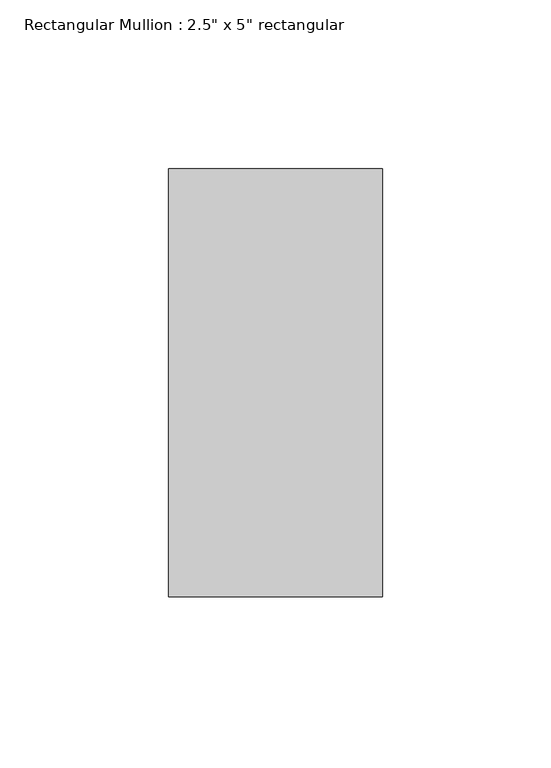
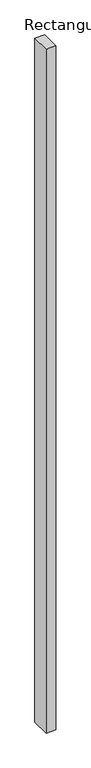
"""IFC4 building model written with IfcOpenShell, lengths in millimetres: member geometry."""

from ifc_helpers import new_model, si_unit, frame, origin, place, context, project, spatial, polyline, outline, extrude, source, transform, mapped, element, save


def member_8a2e7db5(model_context):
    return source(origin(), model_context, "Body", "SweptSolid", [
        extrude(outline(polyline([(0.0, 63.5), (0.0, -63.5), (-63.5, -63.5), (-63.5, 63.5), (0.0, 63.5)])), frame((0.0, 0.0, -4749.8), z_axis=(0.0, 0.0, 1.0), x_axis=(1.0, 0.0, 0.0)), (0.0, 0.0, 1.0), 4749.8),
    ])


if __name__ == "__main__":
    model = new_model("IFC4")
    model_context = context("Model", 3, world=origin())
    ifc_project = project(units=[si_unit("LENGTHUNIT", "METRE", prefix="MILLI")], contexts=[model_context])
    site = spatial("IfcSite", under=ifc_project)
    building = spatial("IfcBuilding", under=site)
    placement = place(None, origin())
    member_shape = member_8a2e7db5(model_context)
    element("IfcMember", 1, ObjectType="Rectangular Mullion : 2.5\" x 5\" rectangular", at=placement, inside=building, context=model_context, shape_type="MappedRepresentation", body=[
        mapped(member_shape, transform((0.0, 0.0, 0.0), x_axis=(1.0, 0.0, 0.0), y_axis=(0.0, 1.0, 0.0), z_axis=(0.0, 0.0, 1.0))),
    ])
    save(model, "model.ifc")

# Revit data of these elements
# Type "Rectangular Mullion : 2.5\" x 5\" rectangular"
#   built-in parameter 1007304 = 0.416667 (stored number, unit not read)
#   built-in parameter 1007301 = 0.104167 (stored number, unit not read)
#   built-in parameter 1007300 = 0.104167 (stored number, unit not read)
# Element 1 (IfcMember, "Rectangular Mullion : 2.5\" x 5\" rectangular")
#   Materials on its faces: "Aluminum"
# Materials
#   "Aluminum": class "Metal", colour RGB 247 247 247, transparency 0, Description = "Aluminum 6061", Cost = 0
